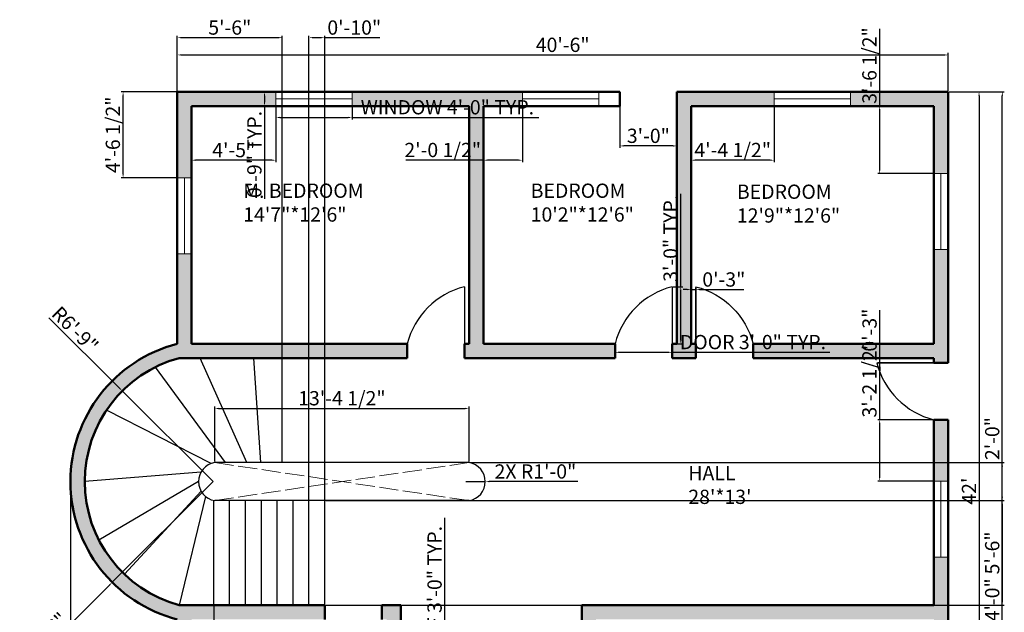
# Model space of a CAD drawing. Units: inches. Extents: x 2291 to 2912, y 1781 to 2517.
# Tile 2 of 2: x 2291 to 2912, y 2143 to 2517. Entities that reach past the tile are written whole.
import ezdxf

# ---------------------------------------------------------------- set-up
doc = ezdxf.new("R2010")
doc.units = ezdxf.units.IN
doc.linetypes.add('ACAD_ISO02W100', pattern=[15, 12, -3])
for name, color, linetype, lineweight in [('A-ANNO-DIMS', 2, 'Continuous', 18), ('A-AREA-IDEN', 7, 'Continuous', 25), ('A-DOOR', 3, 'Continuous', 25), ('A-FLOR-STRS', 7, 'Continuous', 25), ('A-FLOR-STRS-HIDN', 8, 'ACAD_ISO02W100', 13), ('A-GLAZ', 4, 'Continuous', 18), ('A-WALL', 7, 'Continuous', 50)]:
    doc.layers.add(name, color=color, linetype=linetype, lineweight=lineweight)
doc.layers.add('A-WALL-PATT', color=18, linetype='Continuous', lineweight=13, true_color=0x000000)
doc.styles.get("Standard").update_dxf_attribs({"font": 'arial.ttf'})
doc.dimstyles.new('ISO-25', dxfattribs={"dimtxt": 9, "dimasz": 2.5, "dimexe": 1.25, "dimexo": 0.625, "dimtad": 1, "dimlunit": 3, "dimtxsty": 'Standard', "dimcen": 2.5, "dimadec": 0, "dimazin": 0, "dimtfac": 1, "dimtmove": 0, "dimatfit": 3, "dimfxl": 1, "dimarcsym": 0})

# ---------------------------------------------------------------- blocks, each defined once
blk = doc.blocks.new('*D2')
at = {"layer": 'A-ANNO-DIMS', "color": 0, "lineweight": -2, "transparency": 16777216}
for p, q in [((2390.53, 2471.73), (2390.53, 2495.6)), ((2876.53, 2471.73), (2876.53, 2495.6)), ((2393.03, 2494.35), (2874.03, 2494.35))]:
    blk.add_line(p, q, dxfattribs=at)
at = {"layer": 'A-ANNO-DIMS', "color": 0, "transparency": 16777216}
for points in [[(2393.03, 2494.77), (2393.03, 2493.94), (2390.53, 2494.35)], [(2874.03, 2494.77), (2874.03, 2493.94), (2876.53, 2494.35)]]:
    blk.add_solid(points, dxfattribs=at)
at = {"layer": 'Defpoints', "color": 0, "transparency": 16777216}
for p in [(2876.53, 2494.35), (2390.53, 2471.1), (2876.53, 2471.1)]:
    blk.add_point(p, dxfattribs=at)
at = {"layer": 'A-ANNO-DIMS', "color": 0, "transparency": 16777216, "insert": (2633.53, 2499.57), "char_height": 9, "attachment_point": 5}
blk.add_mtext('40\'-6"', dxfattribs=at)
blk = doc.blocks.new('*D3')
at = {"layer": 'A-ANNO-DIMS', "color": 0, "lineweight": -2, "transparency": 16777216}
for p, q in [((2877.16, 2471.1), (2897.25, 2471.1)), ((2896, 2468.6), (2896, 1969.6)), ((2877.16, 1967.1), (2897.25, 1967.1))]:
    blk.add_line(p, q, dxfattribs=at)
at = {"layer": 'A-ANNO-DIMS', "color": 0, "transparency": 16777216}
for points in [[(2895.58, 2468.6), (2896.42, 2468.6), (2896, 2471.1)], [(2895.58, 1969.6), (2896.42, 1969.6), (2896, 1967.1)]]:
    blk.add_solid(points, dxfattribs=at)
at = {"layer": 'Defpoints', "color": 0, "transparency": 16777216}
for p in [(2876.53, 2471.1), (2876.53, 1967.1), (2896, 1967.1)]:
    blk.add_point(p, dxfattribs=at)
at = {"layer": 'A-ANNO-DIMS', "color": 0, "transparency": 16777216, "insert": (2890.86, 2219.1), "char_height": 9, "attachment_point": 5, "rotation": 90}
blk.add_mtext("42'", dxfattribs=at)
blk = doc.blocks.new('WINDOW-48IN')
for p, q in [((9, 48), (0, 48)), ((0, 48), (0, 0)), ((4.5, 0), (4.5, 48)), ((9, 0), (9, 48)), ((0, 0), (9, 0))]:
    blk.add_line(p, q)
blk = doc.blocks.new('DOOR-SINGLE-36IN')
blk.add_line((36, 36), (36, 0))
blk.add_arc((48.43, -12.43), 50, 104.39819, 165.60181)
blk = doc.blocks.new('*D7')
at = {"layer": 'A-ANNO-DIMS', "color": 0, "lineweight": -2, "transparency": 16777216}
for p, q in [((2452.75, 2461.48), (2452.75, 2453.65)), ((2500.75, 2461.48), (2500.75, 2453.65)), ((2455.25, 2454.9), (2498.25, 2454.9)), ((2500.75, 2454.9), (2618.39, 2454.9))]:
    blk.add_line(p, q, dxfattribs=at)
at = {"layer": 'A-ANNO-DIMS', "color": 0, "transparency": 16777216}
for points in [[(2455.25, 2455.32), (2455.25, 2454.48), (2452.75, 2454.9)], [(2498.25, 2455.32), (2498.25, 2454.48), (2500.75, 2454.9)]]:
    blk.add_solid(points, dxfattribs=at)
at = {"layer": 'Defpoints', "color": 0, "transparency": 16777216}
for p in [(2452.75, 2462.1), (2500.75, 2462.1), (2500.75, 2454.9)]:
    blk.add_point(p, dxfattribs=at)
at = {"layer": 'A-ANNO-DIMS', "color": 0, "transparency": 16777216, "insert": (2560.82, 2460.18), "char_height": 9, "attachment_point": 5}
blk.add_mtext('WINDOW 4\'-0" TYP.', dxfattribs=at)
blk = doc.blocks.new('*D8')
at = {"layer": 'A-ANNO-DIMS', "color": 0, "lineweight": -2, "transparency": 16777216}
for p, q in [((2452.12, 2471.1), (2444.3, 2471.1)), ((2445.55, 2468.6), (2445.55, 2464.6)), ((2452.12, 2462.1), (2444.3, 2462.1)), ((2445.55, 2462.1), (2445.55, 2403.49))]:
    blk.add_line(p, q, dxfattribs=at)
at = {"layer": 'A-ANNO-DIMS', "color": 0, "transparency": 16777216}
for points in [[(2445.13, 2468.6), (2445.97, 2468.6), (2445.55, 2471.1)], [(2445.13, 2464.6), (2445.97, 2464.6), (2445.55, 2462.1)]]:
    blk.add_solid(points, dxfattribs=at)
at = {"layer": 'Defpoints', "color": 0, "transparency": 16777216}
for p in [(2452.75, 2471.1), (2445.55, 2462.1), (2452.75, 2462.1)]:
    blk.add_point(p, dxfattribs=at)
at = {"layer": 'A-ANNO-DIMS', "color": 0, "transparency": 16777216, "insert": (2440.33, 2431.55), "char_height": 9, "attachment_point": 5, "rotation": 90}
blk.add_mtext('0\'-9" TYP.', dxfattribs=at)
blk = doc.blocks.new('*D9')
at = {"layer": 'A-ANNO-DIMS', "color": 0, "lineweight": -2, "transparency": 16777216}
for p, q in [((2666.53, 2311.48), (2666.53, 2305.45)), ((2702.53, 2311.48), (2702.53, 2305.45)), ((2669.03, 2306.7), (2700.03, 2306.7)), ((2702.53, 2306.7), (2801.91, 2306.7))]:
    blk.add_line(p, q, dxfattribs=at)
at = {"layer": 'A-ANNO-DIMS', "color": 0, "transparency": 16777216}
for points in [[(2669.03, 2307.12), (2669.03, 2306.28), (2666.53, 2306.7)], [(2700.03, 2307.12), (2700.03, 2306.28), (2702.53, 2306.7)]]:
    blk.add_solid(points, dxfattribs=at)
at = {"layer": 'Defpoints', "color": 0, "transparency": 16777216}
for p in [(2666.53, 2312.1), (2702.53, 2312.1), (2702.53, 2306.7)]:
    blk.add_point(p, dxfattribs=at)
at = {"layer": 'A-ANNO-DIMS', "color": 0, "transparency": 16777216, "insert": (2753.47, 2311.99), "char_height": 9, "attachment_point": 5}
blk.add_mtext('DOOR 3\'-0" TYP.', dxfattribs=at)
blk = doc.blocks.new('*D10')
at = {"layer": 'A-ANNO-DIMS', "color": 0, "lineweight": -2, "transparency": 16777216}
for p, q in [((2707.93, 2348.1), (2707.93, 2406.7)), ((2703.16, 2348.1), (2709.18, 2348.1)), ((2707.93, 2314.6), (2707.93, 2345.6)), ((2703.16, 2312.1), (2709.18, 2312.1))]:
    blk.add_line(p, q, dxfattribs=at)
at = {"layer": 'A-ANNO-DIMS', "color": 0, "transparency": 16777216}
for points in [[(2707.52, 2345.6), (2708.35, 2345.6), (2707.93, 2348.1)], [(2707.52, 2314.6), (2708.35, 2314.6), (2707.93, 2312.1)]]:
    blk.add_solid(points, dxfattribs=at)
at = {"layer": 'Defpoints', "color": 0, "transparency": 16777216}
for p in [(2702.53, 2348.1), (2707.93, 2348.1), (2702.53, 2312.1)]:
    blk.add_point(p, dxfattribs=at)
at = {"layer": 'A-ANNO-DIMS', "color": 0, "transparency": 16777216, "insert": (2702.71, 2378.65), "char_height": 9, "attachment_point": 5, "rotation": 90}
blk.add_mtext('3\'-0" TYP.', dxfattribs=at)
blk = doc.blocks.new('*D11')
at = {"layer": 'A-ANNO-DIMS', "color": 0, "lineweight": -2, "transparency": 16777216}
for p, q in [((2559.13, 2063.1), (2559.13, 2202.28)), ((2563.91, 2063.1), (2557.88, 2063.1)), ((2559.13, 2029.6), (2559.13, 2060.6)), ((2563.91, 2027.1), (2557.88, 2027.1))]:
    blk.add_line(p, q, dxfattribs=at)
at = {"layer": 'A-ANNO-DIMS', "color": 0, "transparency": 16777216}
for points in [[(2558.72, 2060.6), (2559.55, 2060.6), (2559.13, 2063.1)], [(2558.72, 2029.6), (2559.55, 2029.6), (2559.13, 2027.1)]]:
    blk.add_solid(points, dxfattribs=at)
at = {"layer": 'Defpoints', "color": 0, "transparency": 16777216}
for p in [(2559.13, 2063.1), (2564.53, 2063.1), (2564.53, 2027.1)]:
    blk.add_point(p, dxfattribs=at)
at = {"layer": 'A-ANNO-DIMS', "color": 0, "transparency": 16777216, "insert": (2553.91, 2133.94), "char_height": 9, "attachment_point": 5, "rotation": 90}
blk.add_mtext('ENTRY LEAF 3\'-0" TYP.', dxfattribs=at)
blk = doc.blocks.new('*D13')
at = {"layer": 'A-ANNO-DIMS', "color": 0, "lineweight": -2, "transparency": 16777216}
for p, q in [((2877.16, 2471.1), (2911.95, 2471.1)), ((2910.7, 1825.6), (2910.7, 2468.6)), ((2703.66, 1823.1), (2911.95, 1823.1))]:
    blk.add_line(p, q, dxfattribs=at)
at = {"layer": 'A-ANNO-DIMS', "color": 0, "transparency": 16777216}
for points in [[(2910.28, 2468.6), (2911.12, 2468.6), (2910.7, 2471.1)], [(2910.28, 1825.6), (2911.12, 1825.6), (2910.7, 1823.1)]]:
    blk.add_solid(points, dxfattribs=at)
at = {"layer": 'Defpoints', "color": 0, "transparency": 16777216}
for p in [(2876.53, 2471.1), (2910.7, 2471.1), (2703.03, 1823.1)]:
    blk.add_point(p, dxfattribs=at)
at = {"layer": 'A-ANNO-DIMS', "color": 0, "transparency": 16777216, "insert": (2905.48, 2147.1), "char_height": 9, "attachment_point": 5, "rotation": 90}
blk.add_mtext('54\'-0"', dxfattribs=at)
blk = doc.blocks.new('*D14')
at = {"layer": 'A-ANNO-DIMS', "color": 0, "lineweight": -2, "transparency": 16777216}
for p, q in [((2323.2, 2224.48), (2323.2, 1787.69)), ((2876.53, 1966.48), (2876.53, 1787.69)), ((2325.7, 1788.94), (2874.03, 1788.94))]:
    blk.add_line(p, q, dxfattribs=at)
at = {"layer": 'A-ANNO-DIMS', "color": 0, "transparency": 16777216}
for points in [[(2325.7, 1789.35), (2325.7, 1788.52), (2323.2, 1788.94)], [(2874.03, 1789.35), (2874.03, 1788.52), (2876.53, 1788.94)]]:
    blk.add_solid(points, dxfattribs=at)
at = {"layer": 'Defpoints', "color": 0, "transparency": 16777216}
for p in [(2323.2, 2225.1), (2876.53, 1967.1), (2876.53, 1788.94)]:
    blk.add_point(p, dxfattribs=at)
at = {"layer": 'A-ANNO-DIMS', "color": 0, "transparency": 16777216, "insert": (2599.87, 1794.21), "char_height": 9, "attachment_point": 5}
blk.add_mtext('46\'-1 1/2"', dxfattribs=at)
blk = doc.blocks.new('*D17')
at = {"layer": 'A-ANNO-DIMS', "color": 0, "lineweight": -2, "transparency": 16777216}
for p, q in [((2399.53, 2461.48), (2399.53, 2426.69)), ((2452.75, 2461.48), (2452.75, 2426.69)), ((2450.25, 2427.94), (2402.03, 2427.94))]:
    blk.add_line(p, q, dxfattribs=at)
at = {"layer": 'A-ANNO-DIMS', "color": 0, "transparency": 16777216}
for points in [[(2402.03, 2428.35), (2402.03, 2427.52), (2399.53, 2427.94)], [(2450.25, 2428.35), (2450.25, 2427.52), (2452.75, 2427.94)]]:
    blk.add_solid(points, dxfattribs=at)
at = {"layer": 'Defpoints', "color": 0, "transparency": 16777216}
for p in [(2399.53, 2462.1), (2452.75, 2462.1), (2399.53, 2427.94)]:
    blk.add_point(p, dxfattribs=at)
at = {"layer": 'A-ANNO-DIMS', "color": 0, "transparency": 16777216, "insert": (2426.14, 2433.14), "char_height": 9, "attachment_point": 5}
blk.add_mtext('4\'-5"', dxfattribs=at)
blk = doc.blocks.new('*D18')
at = {"layer": 'A-ANNO-DIMS', "color": 0, "lineweight": -2, "transparency": 16777216}
for p, q in [((2583.53, 2461.48), (2583.53, 2426.69)), ((2608.23, 2461.48), (2608.23, 2426.69)), ((2583.53, 2427.94), (2534.73, 2427.94)), ((2605.73, 2427.94), (2586.03, 2427.94))]:
    blk.add_line(p, q, dxfattribs=at)
at = {"layer": 'A-ANNO-DIMS', "color": 0, "transparency": 16777216}
for points in [[(2586.03, 2428.35), (2586.03, 2427.52), (2583.53, 2427.94)], [(2605.73, 2428.35), (2605.73, 2427.52), (2608.23, 2427.94)]]:
    blk.add_solid(points, dxfattribs=at)
at = {"layer": 'Defpoints', "color": 0, "transparency": 16777216}
for p in [(2583.53, 2462.1), (2608.23, 2462.1), (2583.53, 2427.94)]:
    blk.add_point(p, dxfattribs=at)
at = {"layer": 'A-ANNO-DIMS', "color": 0, "transparency": 16777216, "insert": (2557.88, 2433.21), "char_height": 9, "attachment_point": 5}
blk.add_mtext('2\'-0 1/2"', dxfattribs=at)
blk = doc.blocks.new('*D19')
at = {"layer": 'A-ANNO-DIMS', "color": 0, "lineweight": -2, "transparency": 16777216}
for p, q in [((2669.53, 2470.48), (2669.53, 2435.69)), ((2705.53, 2470.48), (2705.53, 2435.69)), ((2703.03, 2436.94), (2672.03, 2436.94))]:
    blk.add_line(p, q, dxfattribs=at)
at = {"layer": 'A-ANNO-DIMS', "color": 0, "transparency": 16777216}
for points in [[(2672.03, 2437.35), (2672.03, 2436.52), (2669.53, 2436.94)], [(2703.03, 2437.35), (2703.03, 2436.52), (2705.53, 2436.94)]]:
    blk.add_solid(points, dxfattribs=at)
at = {"layer": 'Defpoints', "color": 0, "transparency": 16777216}
for p in [(2669.53, 2471.1), (2705.53, 2471.1), (2669.53, 2436.94)]:
    blk.add_point(p, dxfattribs=at)
at = {"layer": 'A-ANNO-DIMS', "color": 0, "transparency": 16777216, "insert": (2687.53, 2442.16), "char_height": 9, "attachment_point": 5}
blk.add_mtext('3\'-0"', dxfattribs=at)
blk = doc.blocks.new('*D20')
at = {"layer": 'A-ANNO-DIMS', "color": 0, "lineweight": -2, "transparency": 16777216}
for p, q in [((2714.53, 2461.48), (2714.53, 2426.69)), ((2766.88, 2461.48), (2766.88, 2426.69)), ((2764.38, 2427.94), (2717.03, 2427.94))]:
    blk.add_line(p, q, dxfattribs=at)
at = {"layer": 'A-ANNO-DIMS', "color": 0, "transparency": 16777216}
for points in [[(2717.03, 2428.35), (2717.03, 2427.52), (2714.53, 2427.94)], [(2764.38, 2428.35), (2764.38, 2427.52), (2766.88, 2427.94)]]:
    blk.add_solid(points, dxfattribs=at)
at = {"layer": 'Defpoints', "color": 0, "transparency": 16777216}
for p in [(2714.53, 2462.1), (2766.88, 2462.1), (2714.53, 2427.94)]:
    blk.add_point(p, dxfattribs=at)
at = {"layer": 'A-ANNO-DIMS', "color": 0, "transparency": 16777216, "insert": (2740.71, 2433.21), "char_height": 9, "attachment_point": 5}
blk.add_mtext('4\'-4 1/2"', dxfattribs=at)
blk = doc.blocks.new('*D23')
at = {"layer": 'A-ANNO-DIMS', "color": 0, "lineweight": -2, "transparency": 16777216}
for p, q in [((2389.91, 2471.1), (2355.12, 2471.1)), ((2356.37, 2419.34), (2356.37, 2468.6)), ((2389.91, 2416.84), (2355.12, 2416.84))]:
    blk.add_line(p, q, dxfattribs=at)
at = {"layer": 'A-ANNO-DIMS', "color": 0, "transparency": 16777216}
for points in [[(2355.95, 2468.6), (2356.79, 2468.6), (2356.37, 2471.1)], [(2355.95, 2419.34), (2356.79, 2419.34), (2356.37, 2416.84)]]:
    blk.add_solid(points, dxfattribs=at)
at = {"layer": 'Defpoints', "color": 0, "transparency": 16777216}
for p in [(2356.37, 2471.1), (2390.53, 2471.1), (2390.53, 2416.84)]:
    blk.add_point(p, dxfattribs=at)
at = {"layer": 'A-ANNO-DIMS', "color": 0, "transparency": 16777216, "insert": (2351.09, 2443.97), "char_height": 9, "attachment_point": 5, "rotation": 90}
blk.add_mtext('4\'-6 1/2"', dxfattribs=at)
blk = doc.blocks.new('*D24')
at = {"layer": 'A-ANNO-DIMS', "color": 0, "lineweight": -2, "transparency": 16777216}
for p, q in [((2833.37, 2462.1), (2833.37, 2510.74)), ((2866.91, 2462.1), (2832.12, 2462.1)), ((2833.37, 2422.01), (2833.37, 2459.6)), ((2866.91, 2419.51), (2832.12, 2419.51))]:
    blk.add_line(p, q, dxfattribs=at)
at = {"layer": 'A-ANNO-DIMS', "color": 0, "transparency": 16777216}
for points in [[(2832.95, 2459.6), (2833.79, 2459.6), (2833.37, 2462.1)], [(2832.95, 2422.01), (2833.79, 2422.01), (2833.37, 2419.51)]]:
    blk.add_solid(points, dxfattribs=at)
at = {"layer": 'Defpoints', "color": 0, "transparency": 16777216}
for p in [(2833.37, 2462.1), (2867.53, 2462.1), (2867.53, 2419.51)]:
    blk.add_point(p, dxfattribs=at)
at = {"layer": 'A-ANNO-DIMS', "color": 0, "transparency": 16777216, "insert": (2828.09, 2487.67), "char_height": 9, "attachment_point": 5, "rotation": 90}
blk.add_mtext('3\'-6 1/2"', dxfattribs=at)
blk = doc.blocks.new('*D27')
at = {"layer": 'A-ANNO-DIMS', "color": 0, "lineweight": -2, "transparency": 16777216}
for p, q in [((2833.37, 2264.1), (2833.37, 2312.74)), ((2866.91, 2264.1), (2832.12, 2264.1)), ((2833.37, 2227.97), (2833.37, 2261.6)), ((2866.91, 2225.47), (2832.12, 2225.47))]:
    blk.add_line(p, q, dxfattribs=at)
at = {"layer": 'A-ANNO-DIMS', "color": 0, "transparency": 16777216}
for points in [[(2832.95, 2261.6), (2833.79, 2261.6), (2833.37, 2264.1)], [(2832.95, 2227.97), (2833.79, 2227.97), (2833.37, 2225.47)]]:
    blk.add_solid(points, dxfattribs=at)
at = {"layer": 'Defpoints', "color": 0, "transparency": 16777216}
for p in [(2833.37, 2264.1), (2867.53, 2264.1), (2867.53, 2225.47)]:
    blk.add_point(p, dxfattribs=at)
at = {"layer": 'A-ANNO-DIMS', "color": 0, "transparency": 16777216, "insert": (2828.09, 2289.67), "char_height": 9, "attachment_point": 5, "rotation": 90}
blk.add_mtext('3\'-2 1/2"', dxfattribs=at)
blk = doc.blocks.new('*D28')
at = {"layer": 'A-ANNO-DIMS', "color": 0, "lineweight": -2, "transparency": 16777216}
for p, q in [((2833.37, 2305.6), (2833.37, 2333.28)), ((2866.91, 2303.1), (2832.12, 2303.1)), ((2833.37, 2300.1), (2833.37, 2303.1)), ((2866.91, 2300.1), (2832.12, 2300.1)), ((2833.37, 2297.6), (2833.37, 2295.1))]:
    blk.add_line(p, q, dxfattribs=at)
at = {"layer": 'A-ANNO-DIMS', "color": 0, "transparency": 16777216}
for points in [[(2832.95, 2305.6), (2833.79, 2305.6), (2833.37, 2303.1)], [(2832.95, 2297.6), (2833.79, 2297.6), (2833.37, 2300.1)]]:
    blk.add_solid(points, dxfattribs=at)
at = {"layer": 'Defpoints', "color": 0, "transparency": 16777216}
for p in [(2833.37, 2303.1), (2867.53, 2303.1), (2867.53, 2300.1)]:
    blk.add_point(p, dxfattribs=at)
at = {"layer": 'A-ANNO-DIMS', "color": 0, "transparency": 16777216, "insert": (2828.15, 2320.69), "char_height": 9, "attachment_point": 5, "rotation": 90}
blk.add_mtext('0\'-3"', dxfattribs=at)
blk = doc.blocks.new('*D29')
at = {"layer": 'A-ANNO-DIMS', "color": 0, "lineweight": -2, "transparency": 16777216}
for p, q in [((2714.53, 2312.73), (2714.53, 2347.52)), ((2717.53, 2312.73), (2717.53, 2347.52)), ((2712.03, 2346.27), (2709.53, 2346.27)), ((2714.53, 2346.27), (2717.53, 2346.27)), ((2720.03, 2346.27), (2747.71, 2346.27))]:
    blk.add_line(p, q, dxfattribs=at)
at = {"layer": 'A-ANNO-DIMS', "color": 0, "transparency": 16777216}
for points in [[(2712.03, 2346.68), (2712.03, 2345.85), (2714.53, 2346.27)], [(2720.03, 2346.68), (2720.03, 2345.85), (2717.53, 2346.27)]]:
    blk.add_solid(points, dxfattribs=at)
at = {"layer": 'Defpoints', "color": 0, "transparency": 16777216}
for p in [(2717.53, 2346.27), (2714.53, 2312.1), (2717.53, 2312.1)]:
    blk.add_point(p, dxfattribs=at)
at = {"layer": 'A-ANNO-DIMS', "color": 0, "transparency": 16777216, "insert": (2735.12, 2351.49), "char_height": 9, "attachment_point": 5}
blk.add_mtext('0\'-3"', dxfattribs=at)
blk = doc.blocks.new('*D31')
at = {"layer": 'A-ANNO-DIMS', "color": 0, "lineweight": -2, "transparency": 16777216}
for p, q in [((2414.12, 2237.73), (2414.12, 2272.52)), ((2574.53, 2237.73), (2574.53, 2272.52)), ((2416.62, 2271.27), (2572.03, 2271.27))]:
    blk.add_line(p, q, dxfattribs=at)
at = {"layer": 'A-ANNO-DIMS', "color": 0, "transparency": 16777216}
for points in [[(2416.62, 2271.68), (2416.62, 2270.85), (2414.12, 2271.27)], [(2572.03, 2271.68), (2572.03, 2270.85), (2574.53, 2271.27)]]:
    blk.add_solid(points, dxfattribs=at)
at = {"layer": 'Defpoints', "color": 0, "transparency": 16777216}
for p in [(2574.53, 2271.27), (2414.12, 2237.1), (2574.53, 2237.1)]:
    blk.add_point(p, dxfattribs=at)
at = {"layer": 'A-ANNO-DIMS', "color": 0, "transparency": 16777216, "insert": (2494.33, 2276.55), "char_height": 9, "attachment_point": 5}
blk.add_mtext('13\'-4 1/2"', dxfattribs=at)
blk = doc.blocks.new('*D32')
at = {"layer": 'A-ANNO-DIMS', "color": 0, "lineweight": -2, "transparency": 16777216}
for p, q in [((2484.16, 2213.1), (2911.95, 2213.1)), ((2910.7, 2210.6), (2910.7, 2149.6)), ((2484.16, 2147.1), (2911.95, 2147.1))]:
    blk.add_line(p, q, dxfattribs=at)
at = {"layer": 'A-ANNO-DIMS', "color": 0, "transparency": 16777216}
for points in [[(2910.28, 2210.6), (2911.12, 2210.6), (2910.7, 2213.1)], [(2910.28, 2149.6), (2911.12, 2149.6), (2910.7, 2147.1)]]:
    blk.add_solid(points, dxfattribs=at)
at = {"layer": 'Defpoints', "color": 0, "transparency": 16777216}
for p in [(2483.53, 2213.1), (2483.53, 2147.1), (2910.7, 2147.1)]:
    blk.add_point(p, dxfattribs=at)
at = {"layer": 'A-ANNO-DIMS', "color": 0, "transparency": 16777216, "insert": (2905.48, 2180.1), "char_height": 9, "attachment_point": 5, "rotation": 90}
blk.add_mtext('5\'-6"', dxfattribs=at)
blk = doc.blocks.new('*D33')
at = {"layer": 'A-ANNO-DIMS', "color": 0, "lineweight": -2, "transparency": 16777216}
for p, q in [((2473.53, 2213.73), (2473.53, 2506.52)), ((2476.03, 2505.27), (2481.03, 2505.27)), ((2483.53, 2213.73), (2483.53, 2506.52)), ((2483.53, 2505.27), (2518.2, 2505.27))]:
    blk.add_line(p, q, dxfattribs=at)
at = {"layer": 'A-ANNO-DIMS', "color": 0, "transparency": 16777216}
for points in [[(2476.03, 2505.68), (2476.03, 2504.85), (2473.53, 2505.27)], [(2481.03, 2505.68), (2481.03, 2504.85), (2483.53, 2505.27)]]:
    blk.add_solid(points, dxfattribs=at)
at = {"layer": 'Defpoints', "color": 0, "transparency": 16777216}
for p in [(2483.53, 2505.27), (2473.53, 2213.1), (2483.53, 2213.1)]:
    blk.add_point(p, dxfattribs=at)
at = {"layer": 'A-ANNO-DIMS', "color": 0, "transparency": 16777216, "insert": (2502.12, 2510.49), "char_height": 9, "attachment_point": 5}
blk.add_mtext('0\'-10"', dxfattribs=at)
blk = doc.blocks.new('*D34')
at = {"layer": 'A-ANNO-DIMS', "color": 0, "lineweight": -2, "transparency": 16777216}
for p, q in [((2910.7, 2237.1), (2910.7, 2264.93)), ((2575.16, 2237.1), (2911.95, 2237.1)), ((2910.7, 2215.6), (2910.7, 2234.6)), ((2575.16, 2213.1), (2911.95, 2213.1))]:
    blk.add_line(p, q, dxfattribs=at)
at = {"layer": 'A-ANNO-DIMS', "color": 0, "transparency": 16777216}
for points in [[(2910.28, 2234.6), (2911.12, 2234.6), (2910.7, 2237.1)], [(2910.28, 2215.6), (2911.12, 2215.6), (2910.7, 2213.1)]]:
    blk.add_solid(points, dxfattribs=at)
at = {"layer": 'Defpoints', "color": 0, "transparency": 16777216}
for p in [(2574.53, 2237.1), (2910.7, 2237.1), (2574.53, 2213.1)]:
    blk.add_point(p, dxfattribs=at)
at = {"layer": 'A-ANNO-DIMS', "color": 0, "transparency": 16777216, "insert": (2905.48, 2252.27), "char_height": 9, "attachment_point": 5, "rotation": 90}
blk.add_mtext('2\'-0"', dxfattribs=at)
blk = doc.blocks.new('*D35')
at = {"layer": 'A-ANNO-DIMS', "color": 0, "lineweight": -2, "transparency": 16777216}
for p, q in [((2390.53, 2312.73), (2390.53, 2506.52)), ((2393.03, 2505.27), (2454.27, 2505.27)), ((2456.77, 2303.73), (2456.77, 2506.52))]:
    blk.add_line(p, q, dxfattribs=at)
at = {"layer": 'A-ANNO-DIMS', "color": 0, "transparency": 16777216}
for points in [[(2393.03, 2505.68), (2393.03, 2504.85), (2390.53, 2505.27)], [(2454.27, 2505.68), (2454.27, 2504.85), (2456.77, 2505.27)]]:
    blk.add_solid(points, dxfattribs=at)
at = {"layer": 'Defpoints', "color": 0, "transparency": 16777216}
for p in [(2456.77, 2505.27), (2390.53, 2312.1), (2456.77, 2303.1)]:
    blk.add_point(p, dxfattribs=at)
at = {"layer": 'A-ANNO-DIMS', "color": 0, "transparency": 16777216, "insert": (2423.65, 2510.49), "char_height": 9, "attachment_point": 5}
blk.add_mtext('5\'-6"', dxfattribs=at)
blk = doc.blocks.new('*D36')
at = {"layer": 'A-ANNO-DIMS', "color": 0, "lineweight": -2, "transparency": 16777216}
for p, q in [((2413.53, 2146.48), (2413.53, 1787.69)), ((2390.53, 2137.48), (2390.53, 1787.69)), ((2393.03, 1788.94), (2411.03, 1788.94)), ((2413.53, 1788.94), (2447.35, 1788.94))]:
    blk.add_line(p, q, dxfattribs=at)
at = {"layer": 'A-ANNO-DIMS', "color": 0, "transparency": 16777216}
for points in [[(2393.03, 1789.35), (2393.03, 1788.52), (2390.53, 1788.94)], [(2411.03, 1789.35), (2411.03, 1788.52), (2413.53, 1788.94)]]:
    blk.add_solid(points, dxfattribs=at)
at = {"layer": 'Defpoints', "color": 0, "transparency": 16777216}
for p in [(2413.53, 2147.1), (2390.53, 2138.1), (2413.53, 1788.94)]:
    blk.add_point(p, dxfattribs=at)
at = {"layer": 'A-ANNO-DIMS', "color": 0, "transparency": 16777216, "insert": (2431.69, 1794.08), "char_height": 9, "attachment_point": 5}
blk.add_mtext('1\'-11"', dxfattribs=at)
blk = doc.blocks.new('*D37')
at = {"layer": 'A-ANNO-DIMS', "color": 0, "lineweight": -2, "transparency": 16777216}
for p, q in [((2413.08, 2225.1), (2349.53, 2161.55)), ((2299.46, 2111.47), (2347.76, 2159.78))]:
    blk.add_line(p, q, dxfattribs=at)
at = {"layer": 'A-ANNO-DIMS', "color": 0, "transparency": 16777216}
blk.add_solid([(2347.47, 2160.08), (2348.06, 2159.49), (2349.53, 2161.55)], dxfattribs=at)
at = {"layer": 'Defpoints', "color": 0, "transparency": 16777216}
for p in [(2413.08, 2225.1), (2349.53, 2161.55)]:
    blk.add_point(p, dxfattribs=at)
at = {"layer": 'A-ANNO-DIMS', "color": 0, "transparency": 16777216, "insert": (2307.71, 2127.11), "char_height": 9, "attachment_point": 5, "rotation": 45.00141}
blk.add_mtext('R7\'-6"', dxfattribs=at)
blk = doc.blocks.new('*D38')
at = {"layer": 'A-ANNO-DIMS', "color": 0, "lineweight": -2, "transparency": 16777216}
for p, q in [((2309.63, 2328.55), (2354.12, 2284.06)), ((2413.08, 2225.1), (2355.89, 2282.29))]:
    blk.add_line(p, q, dxfattribs=at)
at = {"layer": 'A-ANNO-DIMS', "color": 0, "transparency": 16777216}
blk.add_solid([(2354.42, 2284.35), (2353.83, 2283.76), (2355.89, 2282.29)], dxfattribs=at)
at = {"layer": 'Defpoints', "color": 0, "transparency": 16777216}
for p in [(2355.89, 2282.29), (2413.08, 2225.1)]:
    blk.add_point(p, dxfattribs=at)
at = {"layer": 'A-ANNO-DIMS', "color": 0, "transparency": 16777216, "insert": (2325.27, 2320.29), "char_height": 9, "attachment_point": 5, "rotation": 314.99993}
blk.add_mtext('R6\'-9"', dxfattribs=at)
blk = doc.blocks.new('*D39')
at = {"layer": 'A-ANNO-DIMS', "color": 0, "lineweight": -2, "transparency": 16777216}
for p, q in [((2572.54, 2225.1), (2584.7, 2225.1)), ((2642.98, 2225.1), (2587.2, 2225.1))]:
    blk.add_line(p, q, dxfattribs=at)
at = {"layer": 'A-ANNO-DIMS', "color": 0, "transparency": 16777216}
blk.add_solid([(2587.2, 2225.52), (2587.2, 2224.68), (2584.7, 2225.1)], dxfattribs=at)
at = {"layer": 'Defpoints', "color": 0, "transparency": 16777216}
for p in [(2572.54, 2225.1), (2584.7, 2225.1)]:
    blk.add_point(p, dxfattribs=at)
at = {"layer": 'A-ANNO-DIMS', "color": 0, "transparency": 16777216, "insert": (2616.34, 2230.32), "char_height": 9, "attachment_point": 5, "rotation": 359.99765}
blk.add_mtext('2X R1\'-0"', dxfattribs=at)

msp = doc.modelspace()

# ---------------------------------------------------------------- hatches: boundary and pattern name
at = {"layer": 'A-WALL-PATT'}
h = msp.add_hatch(color=256, dxfattribs=at)
h.dxf.hatch_style = 1
h.paths.add_polyline_path([(2608.229, 2471.101), (2500.749, 2471.101), (2500.749, 2462.101), (2574.534, 2462.101), (2574.534, 2312.101), (2571.534, 2312.101), (2571.534, 2303.101), (2666.534, 2303.101), (2666.534, 2312.101), (2583.534, 2312.101), (2583.534, 2462.101), (2608.229, 2462.101)])
h.paths.add_polyline_path([(2452.749, 2471.101), (2390.534, 2471.101), (2390.534, 2416.836), (2399.534, 2416.836), (2399.534, 2462.101), (2452.749, 2462.101)])
h.paths.add_polyline_path([(2399.534, 2368.836), (2390.534, 2368.836), (2390.534, 2312.101, 0.7738955), (2390.534, 2138.101), (2390.534, 2078.695), (2399.534, 2078.695), (2399.534, 2138.101), (2483.534, 2138.101), (2483.534, 2147.101), (2391.712, 2147.101, -0.7629082), (2391.712, 2303.101), (2535.534, 2303.101), (2535.534, 2312.101), (2399.534, 2312.101)])
h.paths.add_polyline_path([(2714.534, 2462.101), (2766.881, 2462.101), (2766.881, 2471.101), (2705.534, 2471.101), (2705.534, 2312.101), (2702.534, 2312.101), (2702.534, 2303.101), (2717.534, 2303.101), (2717.534, 2312.101), (2714.534, 2312.101)])
h.paths.add_polyline_path([(2876.534, 2471.101), (2814.881, 2471.101), (2814.881, 2462.101), (2867.534, 2462.101), (2867.534, 2419.508), (2876.534, 2419.508)])
h.paths.add_polyline_path([(2876.534, 2371.508), (2867.534, 2371.508), (2867.534, 2312.101), (2753.534, 2312.101), (2753.534, 2303.101), (2867.534, 2303.101), (2867.534, 2300.101), (2876.534, 2300.101)])
h.paths.add_polyline_path([(2876.534, 2264.101), (2867.534, 2264.101), (2867.534, 2225.473), (2876.534, 2225.473)])
h.paths.add_polyline_path([(2876.534, 2177.473), (2867.534, 2177.473), (2867.534, 2147.101), (2645.534, 2147.101), (2645.534, 2135.101), (2654.534, 2135.101), (2654.534, 2138.101), (2867.534, 2138.101), (2867.534, 2079.372), (2876.534, 2079.372)])
h.paths.add_polyline_path([(2531.534, 2147.101), (2519.534, 2147.101), (2519.534, 2138.101), (2522.534, 2138.101), (2522.534, 1976.101), (2479.032, 1976.101), (2479.032, 1967.101), (2531.534, 1967.101)])
h.paths.add_polyline_path([(2399.534, 2030.695), (2390.534, 2030.695), (2390.534, 1967.101), (2431.032, 1967.101), (2431.032, 1976.101), (2399.534, 1976.101)])
h.paths.add_polyline_path([(2654.534, 2099.101), (2645.534, 2099.101), (2645.534, 2015.101), (2654.534, 2015.101)])
h.paths.add_polyline_path([(2761.034, 1976.101), (2654.534, 1976.101), (2654.534, 1979.101), (2645.534, 1979.101), (2645.534, 1967.101), (2761.034, 1967.101)])
h.paths.add_polyline_path([(2876.534, 2031.372), (2867.534, 2031.372), (2867.534, 1976.101), (2809.034, 1976.101), (2809.034, 1967.101), (2876.534, 1967.101)])
h.paths.add_polyline_path([(2499.035, 1832.101), (2490.035, 1832.101), (2490.035, 1823.101), (2499.035, 1823.101)])
h.paths.add_polyline_path([(2703.035, 1832.101), (2694.035, 1832.101), (2694.035, 1823.101), (2703.035, 1823.101)])

# ---------------------------------------------------------------- linework, layer by layer
at = {"layer": 'A-DOOR'}
msp.add_line((2717.534, 2348.101), (2717.534, 2312.101), dxfattribs=at)
at = {"layer": 'A-FLOR-STRS'}
for p, q in [((2434.389, 2237.101), (2404.887, 2303.101)), ((2443.29, 2237.101), (2438.713, 2303.101)), ((2456.77, 2237.101), (2456.77, 2303.101)), ((2420.91, 2237.101), (2376.798, 2297.381)), ((2411.803, 2236.477), (2345.984, 2270.255)), ((2574.534, 2237.101), (2414.117, 2237.101)), ((2405.472, 2230.998), (2332.205, 2225.101)), ((2403.947, 2225.101), (2341.147, 2188.137)), ((2405.56, 2219.049), (2357.181, 2166.655)), ((2408.301, 2215.776), (2391.712, 2147.101)), ((2413.534, 2147.101), (2413.534, 2213.101)), ((2574.534, 2213.101), (2414.117, 2213.101)), ((2423.534, 2147.101), (2423.534, 2213.101)), ((2433.534, 2147.101), (2433.534, 2213.101)), ((2443.534, 2147.101), (2443.534, 2213.101)), ((2453.534, 2147.101), (2453.534, 2213.101)), ((2463.534, 2147.101), (2463.534, 2213.101)), ((2473.534, 2147.101), (2473.534, 2213.101)), ((2483.534, 2147.101), (2483.534, 2213.101))]:
    msp.add_line(p, q, dxfattribs=at)
for centre, start, end in [((2416.112, 2225.101), 99.43912, 260.56088), ((2416.112, 2225.101), 99.43912, 260.56088), ((2572.539, 2225.101), 279.43912, 80.56088)]:
    msp.add_arc(centre, 12.165, start, end, dxfattribs=at)
at = {"layer": 'A-FLOR-STRS-HIDN'}
for p, q in [((2414.117, 2213.101), (2574.534, 2237.101)), ((2414.117, 2237.101), (2574.534, 2213.101))]:
    msp.add_line(p, q, dxfattribs=at)
at = {"layer": 'A-WALL'}
for p, q in [((2390.534, 2471.101), (2390.534, 2312.101)), ((2669.534, 2471.101), (2390.534, 2471.101)), ((2669.534, 2471.101), (2669.534, 2462.101)), ((2876.534, 2471.101), (2705.534, 2471.101)), ((2705.534, 2471.101), (2705.534, 2312.101)), ((2876.534, 2300.101), (2876.534, 2471.101)), ((2399.534, 2462.101), (2399.534, 2312.101)), ((2574.534, 2462.101), (2399.534, 2462.101)), ((2574.534, 2462.101), (2574.534, 2312.101)), ((2583.534, 2462.101), (2583.534, 2312.101)), ((2669.534, 2462.101), (2583.534, 2462.101)), ((2867.534, 2462.101), (2714.534, 2462.101)), ((2714.534, 2462.101), (2714.534, 2312.101)), ((2867.534, 2312.101), (2867.534, 2462.101)), ((2535.534, 2312.101), (2399.534, 2312.101)), ((2535.534, 2312.101), (2535.534, 2303.101)), ((2574.534, 2312.101), (2571.534, 2312.101)), ((2571.534, 2312.101), (2571.534, 2303.101)), ((2666.534, 2312.101), (2583.534, 2312.101)), ((2666.534, 2312.101), (2666.534, 2303.101)), ((2705.534, 2312.101), (2702.534, 2312.101)), ((2702.534, 2312.101), (2702.534, 2303.101)), ((2717.534, 2312.101), (2714.534, 2312.101)), ((2717.534, 2312.101), (2717.534, 2303.101)), ((2867.534, 2312.101), (2753.534, 2312.101)), ((2753.534, 2312.101), (2753.534, 2303.101)), ((2535.534, 2303.101), (2391.712, 2303.101)), ((2666.534, 2303.101), (2571.534, 2303.101)), ((2717.534, 2303.101), (2702.534, 2303.101)), ((2867.534, 2303.101), (2753.534, 2303.101)), ((2867.534, 2300.101), (2867.534, 2303.101)), ((2867.534, 2300.101), (2876.534, 2300.101)), ((2867.534, 2147.101), (2867.534, 2264.101)), ((2867.534, 2264.101), (2876.534, 2264.101)), ((2876.534, 1967.101), (2876.534, 2264.101)), ((2483.534, 2147.101), (2391.712, 2147.101)), ((2483.534, 2138.101), (2483.534, 2147.101)), ((2531.534, 2147.101), (2519.534, 2147.101)), ((2519.534, 2138.101), (2519.534, 2147.101)), ((2531.534, 2147.101), (2531.534, 1967.101)), ((2867.534, 2147.101), (2645.534, 2147.101)), ((2645.534, 2135.101), (2645.534, 2147.101))]:
    msp.add_line(p, q, dxfattribs=at)
for radius, start, end in [(89.874, 104.52775, 255.47225), (80.874, 105.319388, 254.680612)]:
    msp.add_arc((2413.078, 2225.101), radius, start, end, dxfattribs=at)

# ---------------------------------------------------------------- block references
at = {"layer": 'A-DOOR'}
for p in [(2535.534, 2312.101), (2666.534, 2312.101)]:
    msp.add_blockref('DOOR-SINGLE-36IN', p, dxfattribs=at)
at = {"layer": 'A-DOOR', "extrusion": (0, 0, -1), "zscale": -1}
msp.add_blockref('DOOR-SINGLE-36IN', (-2753.533, 2312.101), dxfattribs=at)
at = {"layer": 'A-DOOR', "rotation": 90.00000000000539}
msp.add_blockref('DOOR-SINGLE-36IN', (2867.534, 2264.102), dxfattribs=at)
at = {"layer": 'A-GLAZ'}
for p, rotation in [((2452.749, 2471.101), 270.0000000000023), ((2608.229, 2471.101), 270.0000000000025), ((2766.881, 2471.101), 270.0000000000025), ((2399.533, 2416.836), 180), ((2876.533, 2419.508), 180), ((2876.533, 2225.473), 180)]:
    msp.add_blockref('WINDOW-48IN', p, dxfattribs=dict(at, rotation=rotation))

# ---------------------------------------------------------------- texts
at = {"layer": 'A-AREA-IDEN', "attachment_point": 1}
for s, width, insert, char_height in [('M. BEDROOM\\P14\'7"*12\'6"', 125.72554, (2432.132, 2413.174), 9), ('{\\H3.6x;BEDROOM\\P10\'2"*12\'6"}', 44.26515, (2613.343, 2413.174), 2.5), ('{\\H3.6x;BEDROOM\\P12\'9"*12\'6"}', 67.78101, (2743.371, 2412.54), 2.5), ("HALL\\P28'*13'", 108.4565, (2712.744, 2234.993), 9)]:
    msp.add_mtext_dynamic_manual_height_columns(s, width=width, gutter_width=12.5, heights=[0], dxfattribs=dict(at, insert=insert, char_height=char_height))

# ---------------------------------------------------------------- dimensions: what is measured, and where the dimension line sits
at = {"layer": 'A-ANNO-DIMS'}
for base, p1, p2, override, picture, middle in [((2456.77, 2505.266), (2390.534, 2312.101), (2456.77, 2303.101), {"dimdec": 1, "dimlfac": 1, "dimrnd": 0, "dimzin": 1, "dimdsep": 46, "dimlunit": 4, "dimfrac": 2}, '*D35', (2423.652, 2510.487)), ((2483.534, 2505.266), (2473.534, 2213.101), (2483.534, 2213.101), {"dimdec": 1, "dimlfac": 1, "dimrnd": 0, "dimzin": 1, "dimdsep": 46, "dimlunit": 4, "dimfrac": 2}, '*D33', (2502.117, 2510.487)), ((2876.534, 2494.355), (2390.534, 2471.101), (2876.534, 2471.101), {"dimclrd": 0, "dimclre": 0, "dimclrt": 0}, '*D2', (2633.534, 2499.575)), ((2717.534, 2346.266), (2714.534, 2312.101), (2717.534, 2312.101), {"dimdec": 1, "dimlfac": 1, "dimrnd": 0, "dimzin": 1, "dimdsep": 46, "dimlunit": 4, "dimfrac": 2}, '*D29', (2735.121, 2351.49)), ((2574.534, 2271.266), (2414.117, 2237.101), (2574.534, 2237.101), {"dimdec": 1, "dimlfac": 1, "dimrnd": 0, "dimzin": 1, "dimdsep": 46, "dimlunit": 4, "dimfrac": 2}, '*D31', (2494.325, 2276.548)), ((2876.534, 1788.936), (2323.205, 2225.101), (2876.534, 1967.101), {"dimdec": 1, "dimlfac": 1, "dimrnd": 0, "dimzin": 1, "dimdsep": 46, "dimlunit": 4, "dimfrac": 2}, '*D14', (2599.869, 1794.215)), ((2413.534, 1788.936), (2390.534, 2138.101), (2413.534, 2147.101), {"dimdec": 1, "dimlfac": 1, "dimrnd": 0, "dimzin": 1, "dimdsep": 46, "dimlunit": 4, "dimfrac": 2}, '*D36', (2431.693, 1794.08))]:
    dim = msp.add_linear_dim(base=base, p1=p1, p2=p2, dimstyle='ISO-25', override=override, dxfattribs=at)
    dim.commit()
    dim.dimension.update_dxf_attribs({"geometry": picture, "text_midpoint": middle})
for base, p1, p2, angle, override, picture, middle in [((2833.369, 2462.101), (2867.534, 2419.508), (2867.534, 2462.101), 90, {"dimdec": 1, "dimlfac": 1, "dimrnd": 0, "dimzin": 1, "dimdsep": 46, "dimlunit": 4, "dimfrac": 2}, '*D24', (2828.087, 2487.671)), ((2356.369, 2471.101), (2390.534, 2416.836), (2390.534, 2471.101), 90, {"dimdec": 1, "dimlfac": 1, "dimrnd": 0, "dimzin": 1, "dimdsep": 46, "dimlunit": 4, "dimfrac": 2}, '*D23', (2351.09, 2443.969)), ((2669.534, 2436.936), (2705.534, 2471.101), (2669.534, 2471.101), 180, {"dimdec": 1, "dimlfac": 1, "dimrnd": 0, "dimzin": 1, "dimdsep": 46, "dimlunit": 4, "dimfrac": 2}, '*D19', (2687.534, 2442.16)), ((2910.699, 2471.101), (2703.035, 1823.101), (2876.534, 2471.101), 90, {"dimdec": 1, "dimlfac": 1, "dimrnd": 0, "dimzin": 1, "dimdsep": 46, "dimlunit": 4, "dimfrac": 2}, '*D13', (2905.479, 2147.101)), ((2896, 1967.101), (2876.534, 2471.101), (2876.534, 1967.101), 90, {"dimclrd": 0, "dimclre": 0, "dimclrt": 0}, '*D3', (2890.857, 2219.101)), ((2399.534, 2427.936), (2452.749, 2462.101), (2399.534, 2462.101), 180, {"dimdec": 1, "dimlfac": 1, "dimrnd": 0, "dimzin": 1, "dimdsep": 46, "dimlunit": 4, "dimfrac": 2}, '*D17', (2426.141, 2433.138)), ((2583.534, 2427.936), (2608.229, 2462.101), (2583.534, 2462.101), 180, {"dimdec": 1, "dimlfac": 1, "dimrnd": 0, "dimzin": 1, "dimdsep": 46, "dimlunit": 4, "dimfrac": 2}, '*D18', (2557.884, 2433.215)), ((2714.534, 2427.936), (2766.881, 2462.101), (2714.534, 2462.101), 180, {"dimdec": 1, "dimlfac": 1, "dimrnd": 0, "dimzin": 1, "dimdsep": 46, "dimlunit": 4, "dimfrac": 2}, '*D20', (2740.707, 2433.215)), ((2833.369, 2303.101), (2867.534, 2300.101), (2867.534, 2303.101), 90, {"dimdec": 1, "dimlfac": 1, "dimrnd": 0, "dimzin": 1, "dimdsep": 46, "dimlunit": 4, "dimfrac": 2}, '*D28', (2828.145, 2320.689)), ((2833.369, 2264.101), (2867.534, 2225.473), (2867.534, 2264.101), 90, {"dimdec": 1, "dimlfac": 1, "dimrnd": 0, "dimzin": 1, "dimdsep": 46, "dimlunit": 4, "dimfrac": 2}, '*D27', (2828.087, 2289.671)), ((2910.699, 2237.101), (2574.534, 2213.101), (2574.534, 2237.101), 90, {"dimdec": 1, "dimlfac": 1, "dimrnd": 0, "dimzin": 1, "dimdsep": 46, "dimlunit": 4, "dimfrac": 2}, '*D34', (2905.479, 2252.265)), ((2910.699, 2147.101), (2483.534, 2213.101), (2483.534, 2147.101), 90, {"dimdec": 1, "dimlfac": 1, "dimrnd": 0, "dimzin": 1, "dimdsep": 46, "dimlunit": 4, "dimfrac": 2}, '*D32', (2905.479, 2180.101))]:
    dim = msp.add_linear_dim(base=base, p1=p1, p2=p2, angle=angle, dimstyle='ISO-25', override=override, dxfattribs=at)
    dim.commit()
    dim.dimension.update_dxf_attribs({"geometry": picture, "text_midpoint": middle})
for base, p1, p2, angle, text, picture, middle in [((2500.749, 2454.901), (2452.749, 2462.101), (2500.749, 2462.101), 0, 'WINDOW <> TYP.', '*D7', (2560.818, 2460.183)), ((2445.549, 2462.101), (2452.749, 2471.101), (2452.749, 2462.101), 270, '<> TYP.', '*D8', (2440.329, 2431.547)), ((2707.934, 2348.101), (2702.534, 2312.101), (2702.534, 2348.101), 90, '<> TYP.', '*D10', (2702.71, 2378.653)), ((2559.134, 2063.101), (2564.534, 2027.101), (2564.534, 2063.101), 90, 'ENTRY LEAF <> TYP.', '*D11', (2553.91, 2133.941))]:
    dim = msp.add_linear_dim(base=base, p1=p1, p2=p2, angle=angle, text=text, dimstyle='ISO-25', override={"dimdec": 1, "dimlfac": 1, "dimrnd": 0, "dimzin": 1, "dimdsep": 46, "dimlunit": 4, "dimfrac": 2}, dxfattribs=at)
    dim.commit()
    dim.dimension.update_dxf_attribs({"geometry": picture, "text_midpoint": middle})
for mpoint, picture, middle in [((2355.892, 2282.288), '*D38', (2321.58, 2316.6)), ((2349.53, 2161.55), '*D37', (2311.401, 2123.419))]:
    dim = msp.add_radius_dim(center=(2413.078, 2225.101), mpoint=mpoint, dimstyle='ISO-25', override={"dimdec": 1, "dimlfac": 1, "dimrnd": 0, "dimzin": 1, "dimdsep": 46, "dimlunit": 4, "dimfrac": 2}, dxfattribs=at)
    dim.commit()
    dim.dimension.update_dxf_attribs({"geometry": picture, "text_midpoint": middle, "dimtype": 164})
dim = msp.add_linear_dim(base=(2702.534, 2306.701), p1=(2666.534, 2312.101), p2=(2702.534, 2312.101), text='DOOR <> TYP.', dimstyle='ISO-25', override={"dimdec": 1, "dimlfac": 1, "dimrnd": 0, "dimzin": 1, "dimdsep": 46, "dimlunit": 4, "dimfrac": 2}, dxfattribs=at)
dim.commit()
dim.dimension.update_dxf_attribs({"geometry": '*D9', "text_midpoint": (2753.47, 2311.986)})
dim = msp.add_radius_dim(center=(2572.539, 2225.101), mpoint=(2584.703, 2225.101), text='2X <>', dimstyle='ISO-25', override={"dimdec": 1, "dimlfac": 1, "dimrnd": 0, "dimzin": 1, "dimdsep": 46, "dimlunit": 4, "dimfrac": 2}, dxfattribs=at)
dim.commit()
dim.dimension.update_dxf_attribs({"geometry": '*D39', "text_midpoint": (2616.343, 2230.32)})

doc.saveas('drawing.dxf')
